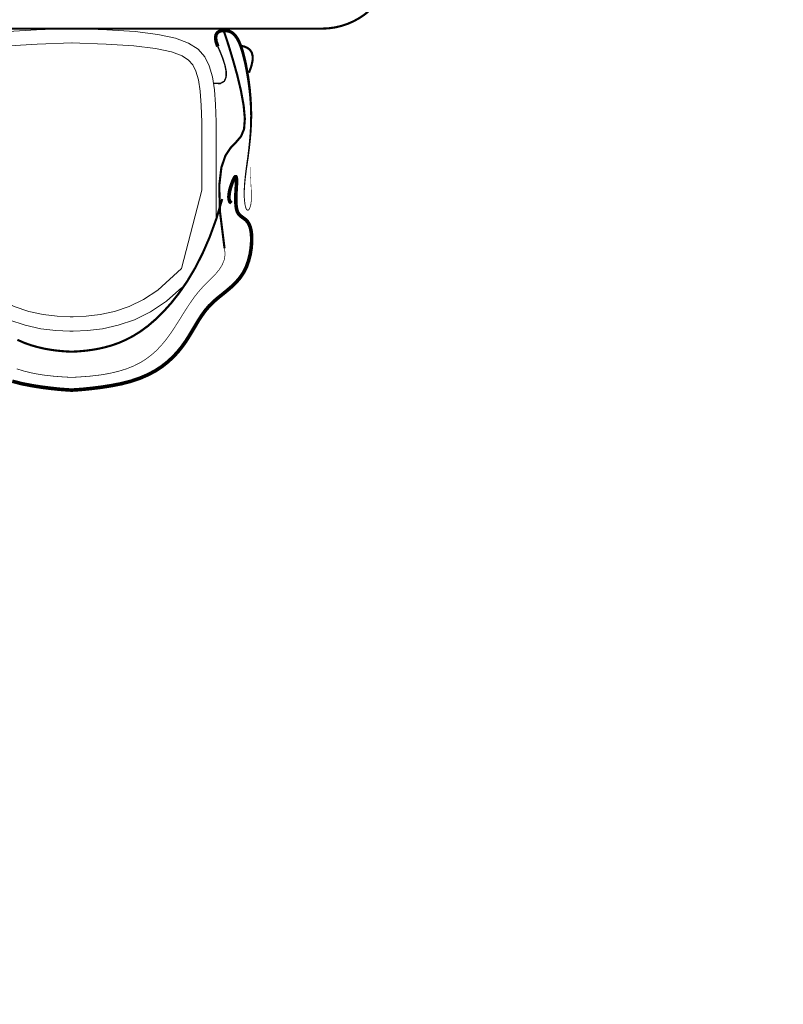
# Model space of a CAD drawing. Units: inches. Extents: x 513 to 1142, y 396 to 927.
# Tile 21 of 31: x 862 to 886, y 691 to 722. Entities that reach past the tile are written whole.
import ezdxf

# ---------------------------------------------------------------- set-up
doc = ezdxf.new("R2010")
doc.units = ezdxf.units.IN
doc.header["$MEASUREMENT"] = 0
doc.linetypes.add('DASHED', pattern=[0.75, 0.5, -0.25])
doc.layers.add('A-ANNO-DIMS', color=2, linetype='DASHED', lineweight=18)
doc.layers.add('furniture', color=92, linetype='Continuous', lineweight=18)
doc.styles.get("Standard").update_dxf_attribs({"font": 'arial.ttf'})
doc.dimstyles.get("Standard").update_dxf_attribs({"dimtxt": 4, "dimasz": 0.18, "dimexe": 0.18, "dimexo": 0.0625, "dimgap": 0.09, "dimtad": 0, "dimtih": 1, "dimtoh": 1, "dimdec": 0, "dimrnd": 6, "dimzin": 0, "dimdsep": 46, "dimlunit": 3, "dimtxsty": 'Standard', "dimcen": 0.09, "dimadec": 0, "dimazin": 0, "dimtfac": 1, "dimtdec": 0, "dimtofl": 0, "dimtmove": 0, "dimatfit": 3, "dimfxl": 1, "dimtolj": 1, "dimtzin": 0, "dimarcsym": 0})

# ---------------------------------------------------------------- blocks, each defined once
blk = doc.blocks.new('ОГ55_на6персон_стол1400х900')
at = {"const_width": 3}
blk.add_lwpolyline([(-600, 279.3), (600, 279.3, -0.414214), (700, 179.3), (700, -520.7, -0.414214), (600, -620.7), (-600, -620.7, -0.414214), (-700, -520.7), (-700, 179.3, -0.414214)], format="xyb", close=True, dxfattribs=at)
for points, const_width in [([(-1193.2, -87.7), (-1196.7, -101.2), (-1199.4, -115.3), (-1201.6, -129.2), (-1203.2, -142.1), (-1204.4, -153.5), (-1205.1, -162.5), (-1205.5, -168.5), (-1205.7, -170.7)], 5), ([(-1175.9, -94), (-1179.3, -105.1), (-1182.2, -117.4), (-1184.5, -130.9), (-1186.2, -145.8), (-1187.4, -162.1), (-1187.8, -170.7)], 1), ([(-1135.3, -94.9), (-1139.6, -104.7), (-1143, -114.3), (-1145.6, -123.7), (-1147.7, -132.7), (-1149.2, -141.4), (-1150.3, -149.3), (-1151, -156.4), (-1151.5, -162.3), (-1151.7, -166.8), (-1151.8, -169.6), (-1151.8, -170.7)], 3), ([(-944.1, -394.1), (-942.1, -391.9), (-938.9, -390.8), (-934.9, -390.6), (-930.3, -391.1), (-925.5, -392), (-920.8, -393.4), (-916.4, -394.9), (-912.7, -396.3), (-909.9, -397.6), (-908, -398.7), (-907.1, -399.6), (-907.1, -400.3), (-908, -400.8), (-909.8, -401.1), (-912.5, -401.2), (-916.1, -401.2), (-920.5, -401), (-925.5, -400.7), (-931, -400.4), (-936.6, -400.2), (-942.2, -400.3), (-947.5, -400.6), (-952.2, -401.3), (-956.2, -402.5), (-959.2, -404.2), (-961.5, -406.4), (-963.4, -408.8), (-965.3, -411.4), (-967.4, -414.1), (-969.9, -416.5), (-973.4, -418.7), (-977.9, -420.5), (-983.8, -421.8), (-990.9, -422.4), (-998.8, -422.4), (-1007.3, -421.7), (-1016.1, -420.3), (-1024.9, -418), (-1033.4, -415), (-1041.3, -411), (-1048.4, -406.2), (-1054.8, -400.7), (-1060.7, -394.6), (-1066.3, -388.1), (-1071.6, -381.6), (-1076.9, -375), (-1082.4, -368.7), (-1088.1, -362.9), (-1094.4, -357.6), (-1101, -352.8), (-1108, -348.2), (-1115.2, -343.9), (-1122.6, -339.5), (-1130.1, -335), (-1137.6, -330.2), (-1145, -324.9), (-1152.3, -319), (-1159.4, -312.4), (-1166.2, -305), (-1172.7, -296.8), (-1178.7, -287.6), (-1184.1, -277.4), (-1189, -266.1), (-1193.2, -253.7), (-1196.7, -240.1), (-1199.4, -226.1), (-1201.6, -212.2), (-1203.2, -199.2), (-1204.4, -187.9), (-1205.1, -178.9), (-1205.5, -172.9), (-1205.7, -170.7)], 5), ([(-1007.2, -384.5), (-1015.9, -385.3), (-1023.6, -384), (-1030.7, -381.1), (-1037.3, -376.9), (-1043.5, -371.8), (-1049.4, -366), (-1055.3, -360), (-1061.3, -354.1), (-1067.5, -348.6), (-1073.9, -343.4), (-1080.6, -338.6), (-1087.4, -334), (-1094.3, -329.5), (-1101.4, -325.1), (-1108.5, -320.7), (-1115.7, -316.1), (-1122.9, -311.4), (-1130, -306.5), (-1137, -301.2), (-1143.8, -295.4), (-1150.3, -289.2), (-1156.4, -282.3), (-1162.1, -274.8), (-1167.3, -266.5), (-1171.9, -257.4), (-1175.9, -247.3), (-1179.3, -236.2), (-1182.2, -224), (-1184.5, -210.5), (-1186.2, -195.6), (-1187.4, -179.3), (-1187.8, -170.7)], 1), ([(-938.3, -381.3), (-966.1, -373), (-991.4, -363.8), (-1014.2, -353.9), (-1034.8, -343.4), (-1053.1, -332.5), (-1069.4, -321.3), (-1083.7, -310), (-1096.1, -298.9), (-1106.8, -287.9), (-1116, -277.2), (-1123.7, -266.7), (-1130.1, -256.4), (-1135.3, -246.4), (-1139.6, -236.6), (-1143, -227), (-1145.6, -217.7), (-1147.7, -208.6), (-1149.2, -200), (-1150.3, -192), (-1151, -185), (-1151.5, -179.1), (-1151.7, -174.6), (-1151.8, -171.7), (-1151.8, -170.7)], 3), ([(-724.9, -375.1), (-732.7, -378.5), (-741.6, -382), (-751, -385), (-760, -386.8), (-767.8, -386.7), (-773.6, -384.2), (-776.8, -378.4), (-776.4, -368.9)], 2), ([(-1007.2, -384.5), (-956.2, -378.1), (-919.4, -377.1), (-894.1, -380.1), (-877.3, -385.9), (-866.4, -393.3), (-858.5, -400.9), (-850.8, -407.5), (-840.7, -411.8), (-826, -412.9), (-807.4, -411.2), (-786.6, -407.4), (-765.2, -402.3), (-744.5, -396.5), (-726.1, -391), (-711.6, -386.3), (-702.6, -383.2)], 3), ([(-761.7, -418.7), (-752.5, -422), (-744.8, -423.7), (-738.5, -423.8), (-733.5, -422.6), (-729.7, -420.1), (-726.9, -416.5), (-725, -411.9), (-723.8, -406.4)], 3)]:
    blk.add_lwpolyline(points, dxfattribs=dict(const_width=const_width))
for points in [[(-966.1, 31.7), (-925.8, 31.2), (-889.9, 31.2), (-858.2, 31.3), (-830.4, 31.2), (-806.3, 30.5), (-785.4, 29), (-767.4, 26.2), (-752.2, 21.8), (-739.4, 15.4), (-728.7, 6.1), (-720.1, -7.2), (-713.2, -25.6), (-708, -50.1), (-704.2, -81.7), (-701.6, -121.6), (-700, -170.7)], [(-1035.7, -17.1), (-925.9, 11.2), (-889.9, 11.2), (-858.2, 11.3), (-830.8, 11.2), (-807.3, 10.5), (-787.6, 9.1), (-771.7, 6.6), (-759.5, 3.1), (-750.6, -1.3), (-744, -7.1), (-738, -16.3), (-732.5, -31.2), (-727.7, -53.4), (-724.1, -83.6), (-721.5, -122.5), (-720, -171.3)], [(-1062.3, -16.7), (-1081.4, -38.1), (-1096.2, -60.3), (-1107.2, -82.9), (-1114.8, -105.5), (-1119.7, -127.5), (-1122.3, -148.6), (-1123.1, -168.3), (-1123.1, -170.7)], [(-1035.7, -17.1), (-1065.6, -50.4), (-1078.8, -70.2), (-1088.7, -90.5), (-1095.5, -110.8), (-1100, -130.9), (-1102.3, -150.3), (-1103.1, -168.6), (-1103.1, -170.3)], [(-1062.3, -324.6), (-1081.4, -303.3), (-1096.2, -281.1), (-1107.2, -258.5), (-1114.8, -235.9), (-1119.7, -213.8), (-1122.3, -192.7), (-1123.1, -173), (-1123.1, -170.7)], [(-1035.7, -324.3), (-1065.6, -291), (-1078.8, -271.1), (-1088.7, -250.9), (-1095.5, -230.5), (-1100, -210.5), (-1102.3, -191.1), (-1103.1, -172.8), (-1103.1, -171.1)], [(-1035.7, -324.3), (-925.9, -352.6), (-889.9, -352.6), (-858.2, -352.7), (-830.8, -352.6), (-807.3, -351.9), (-787.6, -350.4), (-771.7, -348), (-759.5, -344.4), (-750.6, -340), (-744, -334.2), (-738, -325.1), (-732.5, -310.2), (-727.7, -288), (-724.1, -257.8), (-721.5, -218.8), (-720, -170)], [(-966.1, -373), (-925.8, -372.6), (-889.9, -372.6), (-858.2, -372.7), (-830.4, -372.6), (-806.3, -371.9), (-785.4, -370.3), (-767.4, -367.5), (-752.2, -363.2), (-739.4, -356.8), (-728.7, -347.5), (-720.1, -334.1), (-713.2, -315.8), (-708, -291.3), (-704.2, -259.6), (-701.6, -219.8), (-700, -170.7)]]:
    blk.add_lwpolyline(points)
blk.add_lwpolyline([(-724.9, -375.1, 5, 4.91, 0), (-718.1, -372.7, 4.91, 4.84, 0), (-712.8, -372, 4.84, 4.78, 0), (-708.7, -372.6, 4.78, 4.74, 0), (-705.8, -374.3, 4.74, 4.7, 0), (-703.9, -376.9, 4.7, 4.65, 0), (-702.9, -380.1, 4.65, 4.61, 0), (-702.5, -383.6, 4.61, 4.56, 0), (-702.8, -387.1, 4.56, 4.52, 0), (-703.5, -390.5, 4.52, 4.47, 0), (-704.8, -393.6, 4.47, 4.43, 0), (-706.7, -396.6, 4.43, 4.38, 0), (-709.5, -399.3, 4.38, 4.32, 0), (-713.2, -402, 4.32, 4.25, 0), (-717.9, -404.5, 4.25, 4.17, 0), (-723.8, -407, 4.17, 4.07, 0), (-731, -409.4, 4.07, 3.95, 0), (-739.6, -411.7, 3.95, 3.82, 0), (-749.3, -414, 3.82, 3.68, 0), (-760.1, -416, 3.68, 3.53, 0), (-771.6, -417.9, 3.53, 3.37, 0), (-783.7, -419.5, 3.37, 3.21, 0), (-796.2, -420.7, 3.21, 3.05, 0), (-808.8, -421.5, 3.05, 2.88, 0), (-821.4, -421.8, 2.88, 2.72, 0), (-833.8, -421.6, 2.72, 2.57, 0), (-845.8, -420.9, 2.57, 2.41, 0), (-857.4, -419.9, 2.41, 2.27, 0), (-868.5, -418.7, 2.27, 2.13, 0), (-879, -417.4, 2.13, 2, 0), (-888.9, -416, 2, 1.88, 0), (-898, -414.7, 1.88, 1.78, 0), (-906.3, -413.7, 1.78, 1.68, 0), (-913.7, -412.9, 1.68, 1.59, 0), (-920.3, -412.4, 1.59, 1.52, 0), (-926.1, -412.1, 1.52, 1.45, 0), (-931.2, -412, 1.45, 1.4, 0), (-935.6, -412.1, 1.4, 1.35, 0), (-939.4, -412.3, 1.35, 1.3, 0), (-942.6, -412.7, 1.3, 1.27, 0), (-945.3, -413, 1.27, 1.24, 0), (-947.6, -413.5, 1.24, 1.21, 0), (-949.5, -413.9, 1.21, 1.19, 0), (-951, -414.4, 1.19, 1.18, 0), (-952.2, -414.9, 1.18, 1.16, 0), (-953, -415.4, 1.16, 1.15, 0), (-953.6, -416, 1.15, 1.14, 0), (-953.9, -416.5, 1.14, 1.14, 0), (-954, -417, 1.14, 1.13, 0), (-953.9, -417.5, 1.13, 1.12, 0), (-953.6, -418, 1.12, 1.12, 0), (-953.2, -418.5, 1.12, 1.11, 0), (-952.6, -418.9, 1.11, 1.09, 0), (-951.8, -419.4, 1.09, 1.08, 0), (-950.9, -419.8, 1.08, 1.07, 0), (-949.8, -420.2, 1.07, 1.05, 0), (-948.6, -420.6, 1.05, 1.03, 0), (-947.2, -421, 1.03, 1.01, 0), (-945.6, -421.3, 1.01, 0.986, 0), (-943.8, -421.6, 0.986, 0.959, 0), (-941.7, -421.8, 0.959, 0.926, 0), (-939.2, -422, 0.926, 0.889, 0), (-936.3, -422, 0.889, 0.846, 0), (-933, -422, 0.846, 0.796, 0), (-929.1, -422, 0.796, 0.738, 0), (-924.7, -421.8, 0.738, 0.672, 0), (-919.6, -421.5, 0.672, 0.595, 0), (-913.7, -421.2, 0.595, 0.506, 0), (-906.8, -421, 0.506, 0.404, 0), (-898.9, -420.7, 0.404, 0.286, 0), (-889.9, -420.6, 0.286, 0.152, 0), (-879.5, -420.6, 0.152, 0, 0), (-867.8, -420.7, 0, 0, 0)], format="xyseb")
blk = doc.blocks.new('*D137')
at = {"layer": 'A-ANNO-DIMS', "color": 0, "lineweight": -2, "transparency": 16777216}
for p, q in [((839.995, 770.096), (839.995, 401.578)), ((920.995, 770.067), (920.995, 401.578)), ((840.175, 401.758), (875.078, 401.758)), ((920.815, 401.758), (885.913, 401.758))]:
    blk.add_line(p, q, dxfattribs=at)
at = {"layer": 'A-ANNO-DIMS', "color": 0, "transparency": 16777216}
for points in [[(840.175, 401.788), (840.175, 401.728), (839.995, 401.758)], [(920.815, 401.788), (920.815, 401.728), (920.995, 401.758)]]:
    blk.add_solid(points, dxfattribs=at)
at = {"layer": 'Defpoints', "color": 0, "transparency": 16777216}
for p in [(839.995, 770.158), (920.995, 770.13), (920.995, 401.758)]:
    blk.add_point(p, dxfattribs=at)
at = {"layer": 'A-ANNO-DIMS', "color": 0, "transparency": 16777216, "insert": (880.495, 401.758), "char_height": 4, "attachment_point": 5}
blk.add_mtext('\\A1;6\'-9"', dxfattribs=at)
blk = doc.blocks.new('*D149')
at = {"layer": 'A-ANNO-DIMS', "color": 0, "lineweight": -2, "transparency": 16777216}
for p, q in [((840.058, 770.158), (1131.575, 770.158)), ((1131.395, 769.978), (1131.395, 707.791)), ((1131.395, 641.338), (1131.395, 703.526)), ((840.058, 641.158), (1131.575, 641.158))]:
    blk.add_line(p, q, dxfattribs=at)
at = {"layer": 'A-ANNO-DIMS', "color": 0, "transparency": 16777216}
for points in [[(1131.365, 769.978), (1131.425, 769.978), (1131.395, 770.158)], [(1131.365, 641.338), (1131.425, 641.338), (1131.395, 641.158)]]:
    blk.add_solid(points, dxfattribs=at)
at = {"layer": 'Defpoints', "color": 0, "transparency": 16777216}
for p in [(839.995, 770.158), (1131.395, 770.158), (839.995, 641.158)]:
    blk.add_point(p, dxfattribs=at)
at = {"layer": 'A-ANNO-DIMS', "color": 0, "transparency": 16777216, "insert": (1131.395, 705.658), "char_height": 4, "attachment_point": 5}
blk.add_mtext('\\A1;10\'-9"', dxfattribs=at)
blk = doc.blocks.new('*D176')
at = {"layer": 'A-ANNO-DIMS', "color": 0, "lineweight": -2, "transparency": 16777216}
for p, q in [((847.995, 637.221), (847.995, 920.738)), ((891.995, 637.221), (891.995, 920.738)), ((848.175, 920.558), (864.59, 920.558)), ((891.815, 920.558), (875.4, 920.558))]:
    blk.add_line(p, q, dxfattribs=at)
at = {"layer": 'A-ANNO-DIMS', "color": 0, "transparency": 16777216}
for points in [[(848.175, 920.588), (848.175, 920.528), (847.995, 920.558)], [(891.815, 920.588), (891.815, 920.528), (891.995, 920.558)]]:
    blk.add_solid(points, dxfattribs=at)
at = {"layer": 'Defpoints', "color": 0, "transparency": 16777216}
for p in [(891.995, 920.558), (847.995, 637.158), (891.995, 637.158)]:
    blk.add_point(p, dxfattribs=at)
at = {"layer": 'A-ANNO-DIMS', "color": 0, "transparency": 16777216, "insert": (869.995, 920.558), "char_height": 4, "attachment_point": 5}
blk.add_mtext('\\A1;3\'-8"', dxfattribs=at)

msp = doc.modelspace()

# ---------------------------------------------------------------- block references
at = {"layer": 'furniture', "xscale": 0.022676467704094, "yscale": 0.022676467704094, "zscale": 0.022676467704094, "rotation": 90}
msp.add_blockref('ОГ55_на6персон_стол1400х900', (859.781, 737.859), dxfattribs=at)

# ---------------------------------------------------------------- dimensions: what is measured, and where the dimension line sits
at = {"layer": 'A-ANNO-DIMS'}
for base, p1, p2, picture, middle in [((891.995, 920.558), (847.995, 637.158), (891.995, 637.158), '*D176', (869.995, 920.558)), ((920.995, 401.758), (839.995, 770.158), (920.995, 770.13), '*D137', (880.495, 401.758))]:
    dim = msp.add_linear_dim(base=base, p1=p1, p2=p2, dimstyle='Standard', override={"dimdec": 1, "dimlfac": 1, "dimrnd": 0, "dimzin": 1, "dimdsep": 46, "dimlunit": 4, "dimfrac": 2}, dxfattribs=at)
    dim.commit()
    dim.dimension.update_dxf_attribs({"geometry": picture, "text_midpoint": middle})
dim = msp.add_linear_dim(base=(1131.395, 770.158), p1=(839.995, 641.158), p2=(839.995, 770.158), angle=90, dimstyle='Standard', override={"dimdec": 1, "dimlfac": 1, "dimrnd": 0, "dimzin": 1, "dimdsep": 46, "dimlunit": 4, "dimfrac": 2}, dxfattribs=at)
dim.commit()
dim.dimension.update_dxf_attribs({"geometry": '*D149', "text_midpoint": (1131.395, 705.658)})

doc.saveas('drawing.dxf')
